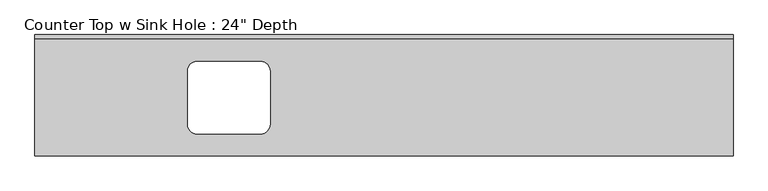
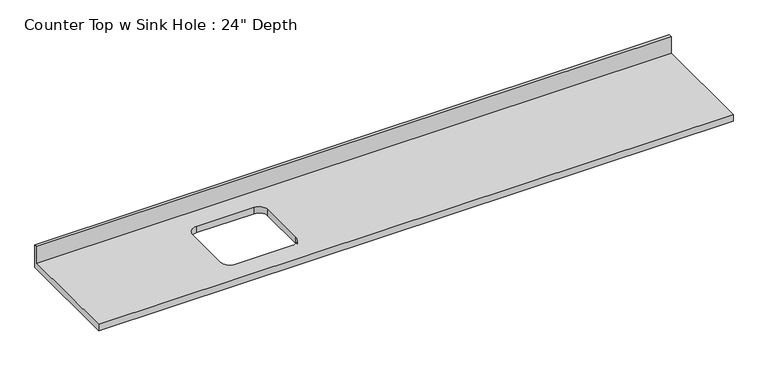
"""IFC4 building model written with IfcOpenShell, lengths in millimetres: furniture geometry."""

from ifc_helpers import new_model, si_unit, frame, origin, place, context, project, spatial, polyline, circle_curve, source, transform, mapped, element, save
from ifc_brep_helpers import plane_surface, revolved_surface, advanced_brep


def furniture_1317d646(model_context):
    return source(origin(), model_context, "Body", "AdvancedBrep", [
        advanced_brep(
        [(-1200.4622951, -635.0, 914.4), (2457.1377049, -635.0, 914.4), (2457.1377049, -19.05, 914.4), (-1200.4622951, -19.05, 914.4), (-349.5622951, -139.7, 914.4), (-19.3622951, -139.7, 914.4), (31.4377049, -190.5, 914.4), (31.4377049, -469.9, 914.4), (-19.3622951, -520.7, 914.4), (-349.5622951, -520.7, 914.4), (-400.3622951, -469.9, 914.4), (-400.3622951, -190.5, 914.4), (2457.1377049, 0.0, 876.3), (2457.1377049, -635.0, 876.3), (-1200.4622951, -635.0, 876.3), (-1200.4622951, 0.0, 876.3), (-19.3622951, -139.7, 876.3), (-349.5622951, -139.7, 876.3), (-400.3622951, -190.5, 876.3), (-400.3622951, -469.9, 876.3), (-349.5622951, -520.7, 876.3), (-19.3622951, -520.7, 876.3), (31.4377049, -469.9, 876.3), (31.4377049, -190.5, 876.3), (-1200.4622951, 0.0, 1016.0), (2457.1377049, 0.0, 1016.0), (-1200.4622951, -19.05, 1016.0), (2457.1377049, -19.05, 1016.0)],
        [
            (0, 1),
            (1, 2),
            (2, 3),
            (3, 0),
            (4, 5),
            (5, 6, circle_curve(frame((-19.3622951, -190.5, 914.4), z_axis=(0.0, 0.0, -1.0), x_axis=(1.0, 0.0, 0.0)), 50.8)),
            (6, 7),
            (7, 8, circle_curve(frame((-19.3622951, -469.9, 914.4), z_axis=(0.0, 0.0, -1.0), x_axis=(1.0, 0.0, 0.0)), 50.8)),
            (8, 9),
            (9, 10, circle_curve(frame((-349.5622951, -469.9, 914.4), z_axis=(0.0, 0.0, -1.0), x_axis=(1.0, 0.0, 0.0)), 50.8)),
            (10, 11),
            (11, 4, circle_curve(frame((-349.5622951, -190.5, 914.4), z_axis=(0.0, 0.0, -1.0), x_axis=(1.0, 0.0, 0.0)), 50.8)),
            (12, 13),
            (13, 14),
            (14, 15),
            (15, 12),
            (16, 17),
            (17, 18, circle_curve(frame((-349.5622951, -190.5, 876.3), z_axis=(0.0, 0.0, 1.0), x_axis=(1.0, 0.0, 0.0)), 50.8)),
            (18, 19),
            (19, 20, circle_curve(frame((-349.5622951, -469.9, 876.3), z_axis=(0.0, 0.0, 1.0), x_axis=(1.0, 0.0, 0.0)), 50.8)),
            (20, 21),
            (21, 22, circle_curve(frame((-19.3622951, -469.9, 876.3), z_axis=(0.0, 0.0, 1.0), x_axis=(1.0, 0.0, 0.0)), 50.8)),
            (22, 23),
            (23, 16, circle_curve(frame((-19.3622951, -190.5, 876.3), z_axis=(0.0, 0.0, 1.0), x_axis=(1.0, 0.0, 0.0)), 50.8)),
            (15, 24),
            (24, 25),
            (25, 12),
            (14, 0),
            (3, 26),
            (26, 24),
            (13, 1),
            (25, 27),
            (27, 2),
            (4, 17),
            (16, 5),
            (11, 18),
            (10, 19),
            (9, 20),
            (8, 21),
            (7, 22),
            (6, 23),
            (26, 27),
        ],
        [
            plane_surface(frame((-1200.4622951, 0.0, 914.4), z_axis=(0.0, 0.0, 1.0), x_axis=(-1.0, 0.0, 0.0))),
            plane_surface(frame((-1200.4622951, 0.0, 876.3), z_axis=(0.0, 0.0, -1.0), x_axis=(1.0, 0.0, 0.0))),
            plane_surface(frame((2457.1377049, 0.0, 914.4), z_axis=(0.0, 1.0, 0.0), x_axis=(0.0, 0.0, -1.0))),
            plane_surface(frame((-1200.4622951, 0.0, 914.4), z_axis=(-1.0, 0.0, 0.0), x_axis=(0.0, 0.0, -1.0))),
            plane_surface(frame((-1200.4622951, -635.0, 914.4), z_axis=(0.0, -1.0, 0.0), x_axis=(0.0, 0.0, -1.0))),
            plane_surface(frame((2457.1377049, -635.0, 914.4), z_axis=(1.0, 0.0, 0.0), x_axis=(0.0, 0.0, -1.0))),
            plane_surface(frame((-19.3622951, -139.7, 914.4), z_axis=(0.0, -1.0, 0.0), x_axis=(0.0, 0.0, -1.0))),
            revolved_surface(polyline([(-298.76229509999996, -190.5, 914.4), (-298.76229509999996, -190.5, 876.3)]), (-349.5622951, -190.5, 876.3), (0.0, 0.0, 1.0)),
            plane_surface(frame((-400.3622951, -190.5, 914.4), z_axis=(1.0, 0.0, 0.0), x_axis=(0.0, 0.0, -1.0))),
            revolved_surface(polyline([(-298.76229509999996, -469.9, 914.4), (-298.76229509999996, -469.9, 876.3)]), (-349.5622951, -469.9, 876.3), (0.0, 0.0, 1.0)),
            plane_surface(frame((-349.5622951, -520.7, 914.4), z_axis=(0.0, 1.0, 0.0), x_axis=(0.0, 0.0, -1.0))),
            revolved_surface(polyline([(31.437704899999996, -469.9, 914.4), (31.437704899999996, -469.9, 876.3)]), (-19.3622951, -469.9, 876.3), (0.0, 0.0, 1.0)),
            plane_surface(frame((31.4377049, -469.9, 914.4), z_axis=(-1.0, 0.0, 0.0), x_axis=(0.0, 0.0, -1.0))),
            revolved_surface(polyline([(31.437704899999996, -190.5, 914.4), (31.437704899999996, -190.5, 876.3)]), (-19.3622951, -190.5, 876.3), (0.0, 0.0, 1.0)),
            plane_surface(frame((-1200.4622951, 0.0, 1016.0), z_axis=(0.0, 0.0, 1.0), x_axis=(0.0, -1.0, 0.0))),
            plane_surface(frame((-1200.4622951, -19.05, 1016.0), z_axis=(0.0, -1.0, 0.0), x_axis=(0.0, 0.0, -1.0))),
        ],
        [
            (0, [[1, 2, 3, 4], [5, 6, 7, 8, 9, 10, 11, 12]]),
            (1, [[13, 14, 15, 16], [17, 18, 19, 20, 21, 22, 23, 24]]),
            (2, [[-16, 25, 26, 27]]),
            (3, [[-15, 28, -4, 29, 30, -25]]),
            (4, [[-1, -28, -14, 31]]),
            (5, [[-13, -27, 32, 33, -2, -31]]),
            (6, [[34, -17, 35, -5]]),
            (7, [[-34, -12, 36, -18]]),
            (8, [[-36, -11, 37, -19]]),
            (9, [[-37, -10, 38, -20]]),
            (10, [[-38, -9, 39, -21]]),
            (11, [[-39, -8, 40, -22]]),
            (12, [[-40, -7, 41, -23]]),
            (13, [[-35, -24, -41, -6]]),
            (14, [[-30, 42, -32, -26]]),
            (15, [[-42, -29, -3, -33]]),
        ],
    ),
    ])


if __name__ == "__main__":
    model = new_model("IFC4")
    model_context = context("Model", 3, world=origin())
    ifc_project = project(units=[si_unit("LENGTHUNIT", "METRE", prefix="MILLI")], contexts=[model_context])
    site = spatial("IfcSite", under=ifc_project)
    building = spatial("IfcBuilding", under=site)
    placement = place(None, origin())
    furniture_shape = furniture_1317d646(model_context)
    element("IfcFurniture", 1, ObjectType="Counter Top w Sink Hole : 24\" Depth", at=placement, inside=building, context=model_context, shape_type="MappedRepresentation", body=[
        mapped(furniture_shape, transform((0.0, 0.0, 0.0), x_axis=(1.0, 0.0, 0.0), y_axis=(0.0, 1.0, 0.0), z_axis=(0.0, 0.0, 1.0))),
    ])
    save(model, "model.ifc")

# Revit data of these elements
# Type "Counter Top w Sink Hole : 24\" Depth"
#   Assembly Code = "C1030400"
#   Counter Thickness = 0' - 1 1/2"
#   Depth = 2' - 1"
#   Height = 3' - 0"
#   Length [instance default] = 8' - 0"
#   Sink Location [instance default] = 2' - 0"
#   Sink Location To Wall [instance default] = 0' - 6"
#   Sink Opening Depth [instance default] = 1' - 3"
#   Sink Opening Width [instance default] = 2' - 3"
#   Counter Top Material = none
#   Default Elevation = 0
# Element 1 (IfcFurniture, "Counter Top w Sink Hole : 24\" Depth")
#   Length = 12' - 0"
#   Sink Location = 3' - 4"
#   Sink Opening Depth = 1' - 2"
#   Sink Opening Width = 1' - 4"
#   Materials on its faces: "Counter Top"
# Materials
#   "Counter Top": class "Wood", colour RGB 226 177 128, transparency 0
